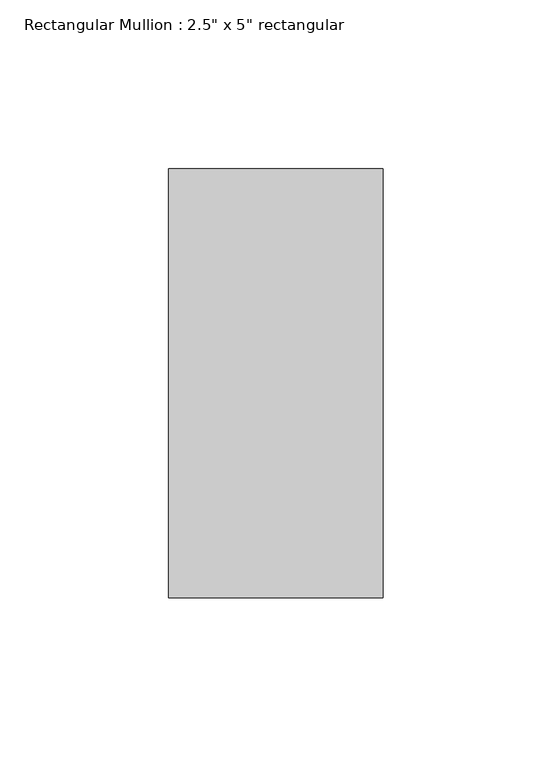
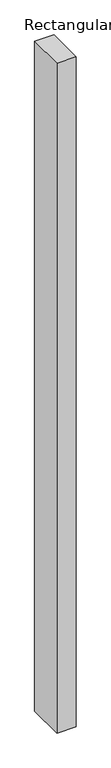
"""IFC4 building model written with IfcOpenShell, lengths in millimetres: member geometry."""

from ifc_helpers import new_model, si_unit, frame, origin, place, context, project, spatial, polyline, outline, extrude, source, transform, mapped, element, save


def member_9bbf3b0c(model_context):
    return source(origin(), model_context, "Body", "SweptSolid", [
        extrude(outline(polyline([(0.0, 63.5), (0.0, -63.5), (-63.5, -63.5), (-63.5, 63.5), (0.0, 63.5)])), frame((0.0, 0.0, -2336.8), z_axis=(0.0, 0.0, 1.0), x_axis=(1.0, 0.0, 0.0)), (0.0, 0.0, 1.0), 2336.8),
    ])


if __name__ == "__main__":
    model = new_model("IFC4")
    model_context = context("Model", 3, world=origin())
    ifc_project = project(units=[si_unit("LENGTHUNIT", "METRE", prefix="MILLI")], contexts=[model_context])
    site = spatial("IfcSite", under=ifc_project)
    building = spatial("IfcBuilding", under=site)
    placement = place(None, origin())
    member_shape = member_9bbf3b0c(model_context)
    element("IfcMember", 1, ObjectType="Rectangular Mullion : 2.5\" x 5\" rectangular", at=placement, inside=building, context=model_context, shape_type="MappedRepresentation", body=[
        mapped(member_shape, transform((0.0, 0.0, 0.0), x_axis=(1.0, 0.0, 0.0), y_axis=(0.0, 1.0, 0.0), z_axis=(0.0, 0.0, 1.0))),
    ])
    save(model, "model.ifc")

# Revit data of these elements
# Type "Rectangular Mullion : 2.5\" x 5\" rectangular"
#   built-in parameter 1007304 = 0.416667 (stored number, unit not read)
#   built-in parameter 1007301 = 0.104167 (stored number, unit not read)
#   built-in parameter 1007300 = 0.104167 (stored number, unit not read)
# Element 1 (IfcMember, "Rectangular Mullion : 2.5\" x 5\" rectangular")
#   Materials on its faces: "Aluminum"
# Materials
#   "Aluminum": class "Metal", colour RGB 247 247 247, transparency 0, Description = "Aluminum 6061", Cost = 0
